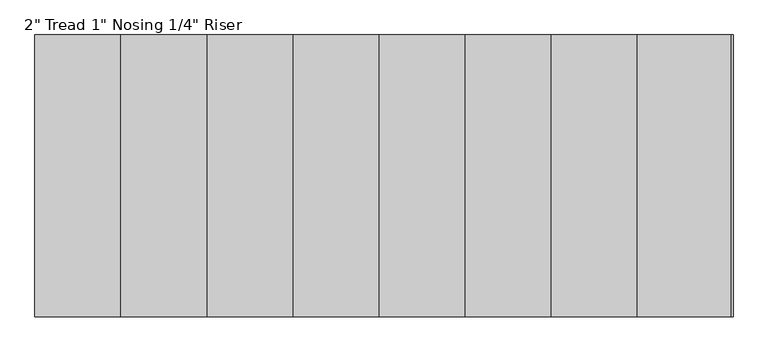
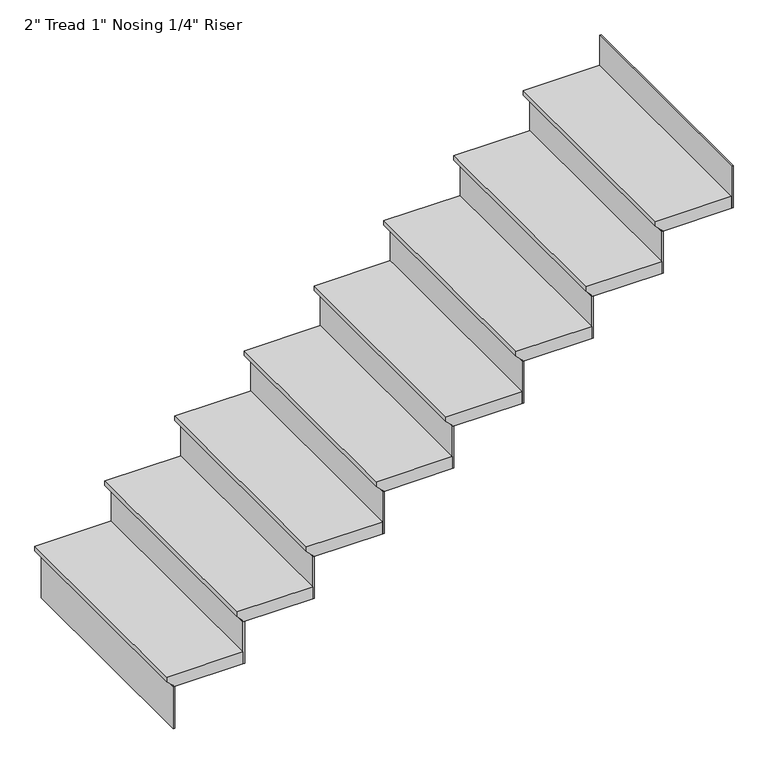
"""IFC4 building model written with IfcOpenShell, lengths in millimetres: stair flight geometry."""

from ifc_helpers import new_model, si_unit, frame, origin, place, context, project, spatial, polyline, outline, extrude, source, transform, mapped, element, save


def stair_flight_f94938bc(model_context):
    return source(origin(), model_context, "Body", "SweptSolid", [
        extrude(outline(polyline([(4978.4, -5173.1473712), (4978.4, -5477.9473712), (4959.35, -5477.9473712), (4933.95, -5452.5473712), (4927.6, -5452.5473712), (4927.6, -5173.1473712), (4978.4, -5173.1473712)])), frame((0.0, -6800.457676, 0.0), z_axis=(0.0, 1.0, 0.0), x_axis=(0.0, 0.0, 1.0)), (0.0, 0.0, 1.0), 914.4),
        extrude(outline(polyline([(-5446.1973712, -6800.457676), (-5452.5473712, -6800.457676), (-5452.5473712, -5886.057676), (-5446.1973712, -5886.057676), (-5446.1973712, -6800.457676)])), frame((0.0, 0.0, 4749.8), z_axis=(0.0, 0.0, 1.0), x_axis=(1.0, 0.0, 0.0)), (0.0, 0.0, 1.0), 177.8),
        extrude(outline(polyline([(-3210.9973712, -6800.457676), (-3217.3473712, -6800.457676), (-3217.3473712, -5886.057676), (-3210.9973712, -5886.057676), (-3210.9973712, -6800.457676)])), frame((0.0, 0.0, 6172.2), z_axis=(0.0, 0.0, 1.0), x_axis=(1.0, 0.0, 0.0)), (0.0, 0.0, 1.0), 177.8),
        extrude(outline(polyline([(-5166.7973712, -6800.457676), (-5173.1473712, -6800.457676), (-5173.1473712, -5886.057676), (-5166.7973712, -5886.057676), (-5166.7973712, -6800.457676)])), frame((0.0, 0.0, 4927.6), z_axis=(0.0, 0.0, 1.0), x_axis=(1.0, 0.0, 0.0)), (0.0, 0.0, 1.0), 177.8),
        extrude(outline(polyline([(5156.2, -4893.7473712), (5156.2, -5198.5473712), (5137.15, -5198.5473712), (5111.75, -5173.1473712), (5105.4, -5173.1473712), (5105.4, -4893.7473712), (5156.2, -4893.7473712)])), frame((0.0, -6800.457676, 0.0), z_axis=(0.0, 1.0, 0.0), x_axis=(0.0, 0.0, 1.0)), (0.0, 0.0, 1.0), 914.4),
        extrude(outline(polyline([(-4887.3973712, -6800.457676), (-4893.7473712, -6800.457676), (-4893.7473712, -5886.057676), (-4887.3973712, -5886.057676), (-4887.3973712, -6800.457676)])), frame((0.0, 0.0, 5105.4), z_axis=(0.0, 0.0, 1.0), x_axis=(1.0, 0.0, 0.0)), (0.0, 0.0, 1.0), 177.8),
        extrude(outline(polyline([(5334.0, -4614.3473712), (5334.0, -4919.1473712), (5314.95, -4919.1473712), (5289.55, -4893.7473712), (5283.2, -4893.7473712), (5283.2, -4614.3473712), (5334.0, -4614.3473712)])), frame((0.0, -6800.457676, 0.0), z_axis=(0.0, 1.0, 0.0), x_axis=(0.0, 0.0, 1.0)), (0.0, 0.0, 1.0), 914.4),
        extrude(outline(polyline([(-4607.9973712, -6800.457676), (-4614.3473712, -6800.457676), (-4614.3473712, -5886.057676), (-4607.9973712, -5886.057676), (-4607.9973712, -6800.457676)])), frame((0.0, 0.0, 5283.2), z_axis=(0.0, 0.0, 1.0), x_axis=(1.0, 0.0, 0.0)), (0.0, 0.0, 1.0), 177.8),
        extrude(outline(polyline([(5511.8, -4334.9473712), (5511.8, -4639.7473712), (5492.75, -4639.7473712), (5467.35, -4614.3473712), (5461.0, -4614.3473712), (5461.0, -4334.9473712), (5511.8, -4334.9473712)])), frame((0.0, -6800.457676, 0.0), z_axis=(0.0, 1.0, 0.0), x_axis=(0.0, 0.0, 1.0)), (0.0, 0.0, 1.0), 914.4),
        extrude(outline(polyline([(-4328.5973712, -6800.457676), (-4334.9473712, -6800.457676), (-4334.9473712, -5886.057676), (-4328.5973712, -5886.057676), (-4328.5973712, -6800.457676)])), frame((0.0, 0.0, 5461.0), z_axis=(0.0, 0.0, 1.0), x_axis=(1.0, 0.0, 0.0)), (0.0, 0.0, 1.0), 177.8),
        extrude(outline(polyline([(5689.6, -4055.5473712), (5689.6, -4360.3473712), (5670.55, -4360.3473712), (5645.15, -4334.9473712), (5638.8, -4334.9473712), (5638.8, -4055.5473712), (5689.6, -4055.5473712)])), frame((0.0, -6800.457676, 0.0), z_axis=(0.0, 1.0, 0.0), x_axis=(0.0, 0.0, 1.0)), (0.0, 0.0, 1.0), 914.4),
        extrude(outline(polyline([(-4049.1973712, -6800.457676), (-4055.5473712, -6800.457676), (-4055.5473712, -5886.057676), (-4049.1973712, -5886.057676), (-4049.1973712, -6800.457676)])), frame((0.0, 0.0, 5638.8), z_axis=(0.0, 0.0, 1.0), x_axis=(1.0, 0.0, 0.0)), (0.0, 0.0, 1.0), 177.8),
        extrude(outline(polyline([(5867.4, -3776.1473712), (5867.4, -4080.9473712), (5848.35, -4080.9473712), (5822.95, -4055.5473712), (5816.6, -4055.5473712), (5816.6, -3776.1473712), (5867.4, -3776.1473712)])), frame((0.0, -6800.457676, 0.0), z_axis=(0.0, 1.0, 0.0), x_axis=(0.0, 0.0, 1.0)), (0.0, 0.0, 1.0), 914.4),
        extrude(outline(polyline([(-3769.7973712, -6800.457676), (-3776.1473712, -6800.457676), (-3776.1473712, -5886.057676), (-3769.7973712, -5886.057676), (-3769.7973712, -6800.457676)])), frame((0.0, 0.0, 5816.6), z_axis=(0.0, 0.0, 1.0), x_axis=(1.0, 0.0, 0.0)), (0.0, 0.0, 1.0), 177.8),
        extrude(outline(polyline([(6045.2, -3496.7473712), (6045.2, -3801.5473712), (6026.15, -3801.5473712), (6000.75, -3776.1473712), (5994.4, -3776.1473712), (5994.4, -3496.7473712), (6045.2, -3496.7473712)])), frame((0.0, -6800.457676, 0.0), z_axis=(0.0, 1.0, 0.0), x_axis=(0.0, 0.0, 1.0)), (0.0, 0.0, 1.0), 914.4),
        extrude(outline(polyline([(-3490.3973712, -6800.457676), (-3496.7473712, -6800.457676), (-3496.7473712, -5886.057676), (-3490.3973712, -5886.057676), (-3490.3973712, -6800.457676)])), frame((0.0, 0.0, 5994.4), z_axis=(0.0, 0.0, 1.0), x_axis=(1.0, 0.0, 0.0)), (0.0, 0.0, 1.0), 177.8),
        extrude(outline(polyline([(6223.0, -3217.3473712), (6223.0, -3522.1473712), (6203.95, -3522.1473712), (6178.55, -3496.7473712), (6172.2, -3496.7473712), (6172.2, -3217.3473712), (6223.0, -3217.3473712)])), frame((0.0, -6800.457676, 0.0), z_axis=(0.0, 1.0, 0.0), x_axis=(0.0, 0.0, 1.0)), (0.0, 0.0, 1.0), 914.4),
    ])


if __name__ == "__main__":
    model = new_model("IFC4")
    model_context = context("Model", 3, world=origin())
    ifc_project = project(units=[si_unit("LENGTHUNIT", "METRE", prefix="MILLI")], contexts=[model_context])
    site = spatial("IfcSite", under=ifc_project)
    building = spatial("IfcBuilding", under=site)
    placement = place(None, origin())
    stair_flight_shape = stair_flight_f94938bc(model_context)
    element("IfcStairFlight", 1, ObjectType="2\" Tread 1\" Nosing 1/4\" Riser", at=placement, inside=building, context=model_context, shape_type="MappedRepresentation", body=[
        mapped(stair_flight_shape, transform((0.0, 0.0, 0.0), x_axis=(1.0, 0.0, 0.0), y_axis=(0.0, 1.0, 0.0), z_axis=(0.0, 0.0, 1.0))),
    ])
    save(model, "model.ifc")
